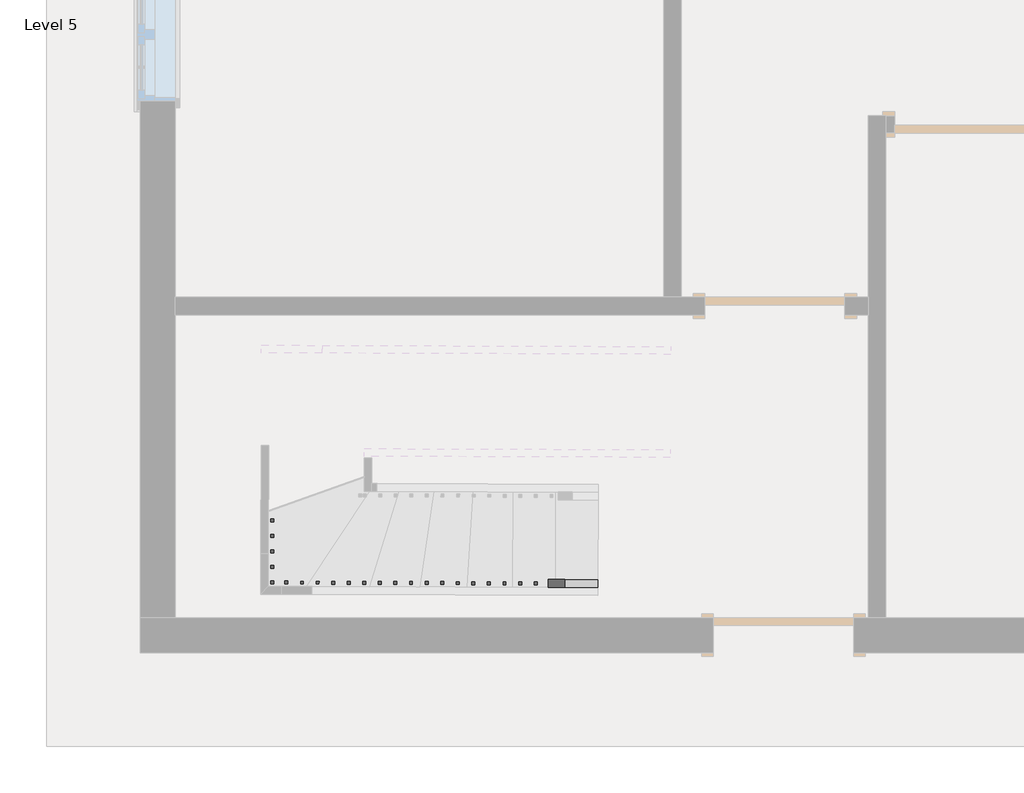
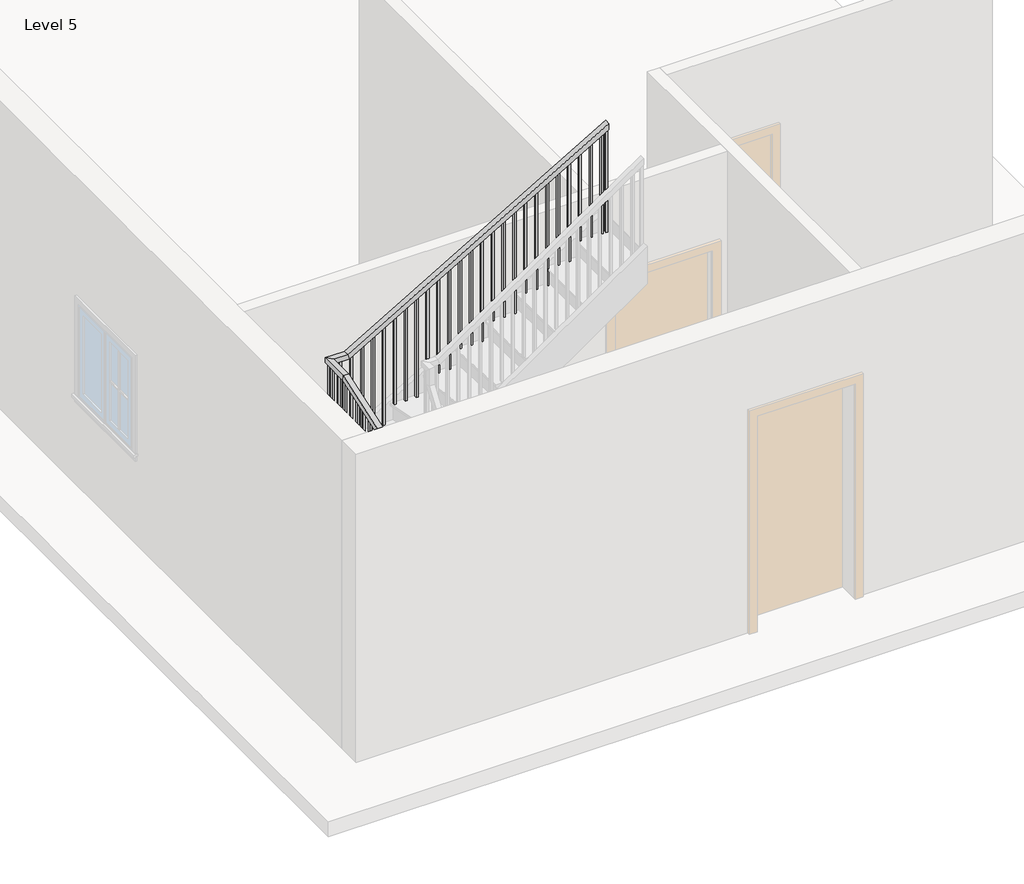
# One storey, part 2 of 3: 1 railing.
"""IFC4 building model written with IfcOpenShell, lengths in millimetres."""

from ifc_helpers import new_model, si_unit, frame, origin, place, context, project, spatial, polyline, outline, extrude, faceted_brep, element, save

model = new_model("IFC4")

# Units and contexts
model_context = context("Model", 3, world=origin())
ifc_project = project(units=[si_unit("LENGTHUNIT", "METRE", prefix="MILLI")], contexts=[model_context])

# Site, building, storey
site = spatial("IfcSite", under=ifc_project)
building = spatial("IfcBuilding", under=site)
storey = spatial("IfcBuildingStorey", under=building, Name="Level 5", Elevation=9601.2)

# Railing
placement = place(None, origin())
element("IfcRailing", 1, ObjectType="Handrail - Rectangular", at=placement, inside=storey, context=model_context, shape_type="SolidModel", body=[
    faceted_brep([(-2342.0274141, -4826.0015756, 10684.9333333), (-2342.0274141, -4826.0015756, 10627.3375993), (-2341.8555281, -4775.2018664, 10627.3375993), (-2341.8555281, -4775.2018664, 10684.9333333), (-4375.5150225, -4819.1210645, 11771.3704289), (-4388.2346185, -4819.0780265, 11720.5704289), (-4388.0627326, -4768.2783173, 11720.5704289), (-4375.3431366, -4768.3213553, 11771.3704289), (-4491.7270905, -4818.7278493, 11771.3704289), (-4491.7270905, -4818.7278493, 11720.5704289), (-4440.7554953, -4768.100026, 11720.5704289), (-4440.7554953, -4768.100026, 11771.3704289), (-4491.153576, -4649.2296115, 11771.3704289), (-4491.1254156, -4640.9069784, 11720.5704289), (-4440.3257064, -4641.0788644, 11720.5704289), (-4440.3538668, -4649.4014974, 11771.3704289), (-4487.5712496, -3590.4977417, 12127.849629), (-4487.5430892, -3582.1751086, 12077.049629), (-4436.74338, -3582.3469946, 12077.049629), (-4436.7715404, -3590.6696276, 12127.849629), (-4486.5726753, -3295.3759891, 12127.849629), (-4486.5726753, -3295.3759891, 12077.049629), (-4435.9448521, -3346.3475843, 12077.049629), (-4435.9448521, -3346.3475843, 12127.849629), (-4306.8228358, -3295.9841909, 12127.849629), (-4292.9867911, -3296.0310065, 12077.049629), (-4293.1586771, -3346.8307157, 12077.049629), (-4306.9947217, -3346.7839001, 12127.849629), (-1866.6470501, -3304.2407725, 13563.6), (-1866.8189361, -3355.0404817, 13563.6), (-1866.8189361, -3355.0404817, 13504.6591495), (-1866.6470501, -3304.2407725, 13504.6591495)], [[[0, 1, 2, 3]], [[1, 0, 4, 5]], [[2, 1, 5, 6]], [[3, 2, 6, 7]], [[0, 3, 7, 4]], [[5, 4, 8, 9]], [[6, 5, 9, 10]], [[7, 6, 10, 11]], [[4, 7, 11, 8]], [[9, 8, 12, 13]], [[10, 9, 13, 14]], [[11, 10, 14, 15]], [[8, 11, 15, 12]], [[13, 12, 16, 17]], [[14, 13, 17, 18]], [[15, 14, 18, 19]], [[12, 15, 19, 16]], [[17, 16, 20, 21]], [[18, 17, 21, 22]], [[19, 18, 22, 23]], [[16, 19, 23, 20]], [[21, 20, 24, 25]], [[22, 21, 25, 26]], [[23, 22, 26, 27]], [[20, 23, 27, 24]], [[28, 29, 30, 31]], [[25, 24, 28, 31]], [[26, 25, 31, 30]], [[27, 26, 30, 29]], [[24, 27, 29, 28]]]),
    extrude(outline(polyline([(234.2042864, 19.05), (1221.3020607, 19.05), (1221.3020607, 0.0), (222.9957135, 0.0), (234.2042864, 19.05)])), frame((-1911.7805866, -3339.0132586, 13701.1687274), z_axis=(0.0033835818014388316, 0.9999942756707125, 0.0), x_axis=(0.0, 0.0, -1.0)), (0.0, 0.0, 1.0), 19.05),
    extrude(outline(polyline([(234.2042864, 19.0499999), (1161.5230057, 19.0499999), (1161.5230057, 0.0), (222.9957136, 0.0), (234.2042864, 19.0499999)])), frame((-2013.3800051, -3338.6694867, 13641.3896724), z_axis=(0.0033835818014388316, 0.9999942756707125, 0.0), x_axis=(0.0, 0.0, -1.0)), (0.0, 0.0, 1.0), 19.05),
    extrude(outline(polyline([(234.2042864, 19.0499999), (1101.7439506, 19.0499999), (1101.7439506, 0.0), (222.9957136, 0.0), (234.2042864, 19.0499999)])), frame((-2114.9794235, -3338.3257147, 13581.6106173), z_axis=(0.0033835818014388316, 0.9999942756707125, 0.0), x_axis=(0.0, 0.0, -1.0)), (0.0, 0.0, 1.0), 19.05),
    extrude(outline(polyline([(234.2042864, 19.0499999), (1211.2982289, 19.0499999), (1211.2982289, 0.0), (222.9957135, 0.0), (234.2042864, 19.0499999)])), frame((-2216.5788419, -3337.9819428, 13521.8315622), z_axis=(0.0033835818014388316, 0.9999942756707125, 0.0), x_axis=(0.0, 0.0, -1.0)), (0.0, 0.0, 1.0), 19.05),
    extrude(outline(polyline([(234.2042864, 19.0499999), (1151.5191739, 19.0499999), (1151.5191739, 0.0), (222.9957136, 0.0), (234.2042864, 19.0499999)])), frame((-2318.1782603, -3337.6381709, 13462.0525072), z_axis=(0.0033835818014388316, 0.9999942756707125, 0.0), x_axis=(0.0, 0.0, -1.0)), (0.0, 0.0, 1.0), 19.05),
    extrude(outline(polyline([(234.2042864, 19.0499999), (1261.0734521, 19.0499999), (1261.0734521, 0.0), (222.9957136, 0.0), (234.2042864, 19.0499999)])), frame((-2419.7776787, -3337.294399, 13402.2734521), z_axis=(0.0033835818014388316, 0.9999942756707125, 0.0), x_axis=(0.0, 0.0, -1.0)), (0.0, 0.0, 1.0), 19.05),
    extrude(outline(polyline([(234.2042864, 19.0499999), (1201.294397, 19.0499999), (1201.294397, 0.0), (222.9957136, 0.0), (234.2042864, 19.0499999)])), frame((-2521.3770971, -3336.9506271, 13342.494397), z_axis=(0.0033835818014388316, 0.9999942756707125, 0.0), x_axis=(0.0, 0.0, -1.0)), (0.0, 0.0, 1.0), 19.05),
    extrude(outline(polyline([(234.2042864, 19.05), (1141.515342, 19.05), (1141.515342, 0.0), (222.9957136, 0.0), (234.2042864, 19.05)])), frame((-2622.9765155, -3336.6068552, 13282.715342), z_axis=(0.0033835818014388316, 0.9999942756707125, 0.0), x_axis=(0.0, 0.0, -1.0)), (0.0, 0.0, 1.0), 19.05),
    extrude(outline(polyline([(234.2042864, 19.05), (1251.0696202, 19.05), (1251.0696202, 0.0), (222.9957136, 0.0), (234.2042864, 19.05)])), frame((-2724.5759339, -3336.2630833, 13222.9362869), z_axis=(0.0033835818014388316, 0.9999942756707125, 0.0), x_axis=(0.0, 0.0, -1.0)), (0.0, 0.0, 1.0), 19.05),
    extrude(outline(polyline([(234.2042864, 19.05), (1191.2905651, 19.05), (1191.2905651, 0.0), (222.9957136, 0.0), (234.2042864, 19.05)])), frame((-2826.1753523, -3335.9193114, 13163.1572318), z_axis=(0.0033835818014388316, 0.9999942756707125, 0.0), x_axis=(0.0, 0.0, -1.0)), (0.0, 0.0, 1.0), 19.05),
    extrude(outline(polyline([(234.2042865, 19.05), (1131.5115101, 19.05), (1131.5115101, 0.0), (222.9957136, 0.0), (234.2042865, 19.05)])), frame((-2927.7747707, -3335.5755395, 13103.3781768), z_axis=(0.0033835818014388316, 0.9999942756707125, 0.0), x_axis=(0.0, 0.0, -1.0)), (0.0, 0.0, 1.0), 19.05),
    extrude(outline(polyline([(234.2042864, 19.05), (1241.0657884, 19.05), (1241.0657884, 0.0), (222.9957136, 0.0), (234.2042864, 19.05)])), frame((-3029.3741891, -3335.2317675, 13043.5991217), z_axis=(0.0033835818014388316, 0.9999942756707125, 0.0), x_axis=(0.0, 0.0, -1.0)), (0.0, 0.0, 1.0), 19.05),
    extrude(outline(polyline([(234.2042864, 19.05), (1181.2867333, 19.05), (1181.2867333, 0.0), (222.9957136, 0.0), (234.2042864, 19.05)])), frame((-3130.9736075, -3334.8879956, 12983.8200666), z_axis=(0.0033835818014388316, 0.9999942756707125, 0.0), x_axis=(0.0, 0.0, -1.0)), (0.0, 0.0, 1.0), 19.05),
    extrude(outline(polyline([(234.2042865, 19.0499999), (1121.5076783, 19.0499999), (1121.5076783, 0.0), (222.9957136, 0.0), (234.2042865, 19.0499999)])), frame((-3232.573026, -3334.5442237, 12924.0410116), z_axis=(0.0033835818014388316, 0.9999942756707125, 0.0), x_axis=(0.0, 0.0, -1.0)), (0.0, 0.0, 1.0), 19.05),
    extrude(outline(polyline([(234.2042864, 19.0499999), (1231.0619565, 19.0499999), (1231.0619565, 0.0), (222.9957136, 0.0), (234.2042864, 19.0499999)])), frame((-3334.1724444, -3334.2004518, 12864.2619565), z_axis=(0.0033835818014388316, 0.9999942756707125, 0.0), x_axis=(0.0, 0.0, -1.0)), (0.0, 0.0, 1.0), 19.05),
    extrude(outline(polyline([(234.2042864, 19.0499999), (1171.2829014, 19.0499999), (1171.2829014, 0.0), (222.9957136, 0.0), (234.2042864, 19.0499999)])), frame((-3435.7718628, -3333.8566799, 12804.4829014), z_axis=(0.0033835818014388316, 0.9999942756707125, 0.0), x_axis=(0.0, 0.0, -1.0)), (0.0, 0.0, 1.0), 19.05),
    extrude(outline(polyline([(234.2042864, 19.0499999), (1111.5038463, 19.0499999), (1111.5038463, 0.0), (222.9957135, 0.0), (234.2042864, 19.0499999)])), frame((-3537.3712812, -3333.512908, 12744.7038463), z_axis=(0.0033835818014388316, 0.9999942756707125, 0.0), x_axis=(0.0, 0.0, -1.0)), (0.0, 0.0, 1.0), 19.05),
    extrude(outline(polyline([(234.2042864, 19.0499999), (1221.0581246, 19.0499999), (1221.0581246, 0.0), (222.9957136, 0.0), (234.2042864, 19.0499999)])), frame((-3638.9706996, -3333.1691361, 12684.9247913), z_axis=(0.0033835818014388316, 0.9999942756707125, 0.0), x_axis=(0.0, 0.0, -1.0)), (0.0, 0.0, 1.0), 19.05),
    extrude(outline(polyline([(234.2042864, 19.0499999), (1161.2790695, 19.0499999), (1161.2790695, 0.0), (222.9957136, 0.0), (234.2042864, 19.0499999)])), frame((-3740.570118, -3332.8253642, 12625.1457362), z_axis=(0.0033835818014388316, 0.9999942756707125, 0.0), x_axis=(0.0, 0.0, -1.0)), (0.0, 0.0, 1.0), 19.05),
    extrude(outline(polyline([(234.2042864, 19.05), (1101.5000144, 19.05), (1101.5000144, 0.0), (222.9957135, 0.0), (234.2042864, 19.05)])), frame((-3842.1695364, -3332.4815923, 12565.3666811), z_axis=(0.0033835818014388316, 0.9999942756707125, 0.0), x_axis=(0.0, 0.0, -1.0)), (0.0, 0.0, 1.0), 19.05),
    extrude(outline(polyline([(234.2042864, 19.05), (1211.0542928, 19.05), (1211.0542928, 0.0), (222.9957136, 0.0), (234.2042864, 19.05)])), frame((-3943.7689548, -3332.1378203, 12505.5876261), z_axis=(0.0033835818014388316, 0.9999942756707125, 0.0), x_axis=(0.0, 0.0, -1.0)), (0.0, 0.0, 1.0), 19.05),
    extrude(outline(polyline([(234.2042864, 19.05), (1151.2752377, 19.05), (1151.2752377, 0.0), (222.9957136, 0.0), (234.2042864, 19.05)])), frame((-4045.3683732, -3331.7940484, 12445.808571), z_axis=(0.0033835818014388316, 0.9999942756707125, 0.0), x_axis=(0.0, 0.0, -1.0)), (0.0, 0.0, 1.0), 19.05),
    extrude(outline(polyline([(234.2042864, 19.05), (1091.4961826, 19.05), (1091.4961826, 0.0), (222.9957136, 0.0), (234.2042864, 19.05)])), frame((-4146.9677916, -3331.4502765, 12386.0295159), z_axis=(0.0033835818014388316, 0.9999942756707125, 0.0), x_axis=(0.0, 0.0, -1.0)), (0.0, 0.0, 1.0), 19.05),
    extrude(outline(polyline([(234.2042865, 19.05), (1031.7171276, 19.05), (1031.7171276, 0.0), (222.9957136, 0.0), (234.2042865, 19.05)])), frame((-4248.56721, -3331.1065046, 12326.2504609), z_axis=(0.0033835818014388316, 0.9999942756707125, 0.0), x_axis=(0.0, 0.0, -1.0)), (0.0, 0.0, 1.0), 19.05),
    extrude(outline(polyline([(-4369.1520622, -3311.6483845), (-4350.1021712, -3311.7128418), (-4350.1666284, -3330.7627327), (-4369.2165194, -3330.6982755), (-4369.1520622, -3311.6483845)])), frame((0.0, 0.0, 11294.5333333), z_axis=(0.0, 0.0, 1.0), x_axis=(1.0, 0.0, 0.0)), (0.0, 0.0, 1.0), 782.5162957),
    extrude(outline(polyline([(-4470.9856602, -3380.5147968), (-4470.921203, -3361.4649058), (-4451.871312, -3361.5293631), (-4451.9357693, -3380.579254), (-4470.9856602, -3380.5147968)])), frame((0.0, 0.0, 11294.5333333), z_axis=(0.0, 0.0, 1.0), x_axis=(1.0, 0.0, 0.0)), (0.0, 0.0, 1.0), 782.5162957),
    extrude(outline(polyline([(-4471.3294321, -3482.1142152), (-4471.2649749, -3463.0643242), (-4452.215084, -3463.1287815), (-4452.2795412, -3482.1786724), (-4471.3294321, -3482.1142152)])), frame((0.0, 0.0, 11125.2), z_axis=(0.0, 0.0, 1.0), x_axis=(1.0, 0.0, 0.0)), (0.0, 0.0, 1.0), 951.849629),
    extrude(outline(polyline([(-4471.6732041, -3583.7136336), (-4471.6087468, -3564.6637426), (-4452.5588559, -3564.7281999), (-4452.6233131, -3583.7780908), (-4471.6732041, -3583.7136336)])), frame((0.0, 0.0, 11125.2), z_axis=(0.0, 0.0, 1.0), x_axis=(1.0, 0.0, 0.0)), (0.0, 0.0, 1.0), 951.849629),
    extrude(outline(polyline([(231.8070867, 19.0499999), (1148.9478489, 19.0499999), (1148.9478489, 0.0), (225.3929132, 0.0), (231.8070867, 19.0499999)])), frame((-4452.9026278, -3666.3276183, 12274.1478489), z_axis=(-0.9999942756707125, 0.003383581801438912, 0.0), x_axis=(0.0, 0.0, -1.0)), (0.0, 0.0, 1.0), 19.05),
    extrude(outline(polyline([(231.8070868, 19.0499999), (1114.7389237, 19.0499999), (1114.7389237, 0.0), (225.3929133, 0.0), (231.8070868, 19.0499999)])), frame((-4453.2463997, -3767.9270367, 12239.9389237), z_axis=(-0.9999942756707125, 0.003383581801438912, 0.0), x_axis=(0.0, 0.0, -1.0)), (0.0, 0.0, 1.0), 19.05),
    extrude(outline(polyline([(231.8070867, 19.0499999), (1080.5299984, 19.0499999), (1080.5299984, 0.0), (225.3929132, 0.0), (231.8070867, 19.0499999)])), frame((-4453.5901716, -3869.5264551, 12205.7299984), z_axis=(-0.9999942756707125, 0.003383581801438912, 0.0), x_axis=(0.0, 0.0, -1.0)), (0.0, 0.0, 1.0), 19.05),
    extrude(outline(polyline([(231.8070867, 19.05), (1215.6544064, 19.05), (1215.6544064, 0.0), (225.3929132, 0.0), (231.8070867, 19.05)])), frame((-4453.9339435, -3971.1258735, 12171.5210731), z_axis=(-0.9999942756707125, 0.003383581801438912, 0.0), x_axis=(0.0, 0.0, -1.0)), (0.0, 0.0, 1.0), 19.05),
    extrude(outline(polyline([(231.8070868, 19.05), (1181.4454812, 19.05), (1181.4454812, 0.0), (225.3929133, 0.0), (231.8070868, 19.05)])), frame((-4454.2777154, -4072.7252919, 12137.3121479), z_axis=(-0.9999942756707125, 0.003383581801438912, 0.0), x_axis=(0.0, 0.0, -1.0)), (0.0, 0.0, 1.0), 19.05),
    extrude(outline(polyline([(231.8070867, 19.05), (1147.2365559, 19.05), (1147.2365559, 0.0), (225.3929132, 0.0), (231.8070867, 19.05)])), frame((-4454.6214873, -4174.3247103, 12103.1032226), z_axis=(-0.9999942756707125, 0.003383581801438912, 0.0), x_axis=(0.0, 0.0, -1.0)), (0.0, 0.0, 1.0), 19.05),
    extrude(outline(polyline([(231.8070868, 19.05), (1113.0276307, 19.05), (1113.0276307, 0.0), (225.3929133, 0.0), (231.8070868, 19.05)])), frame((-4454.9652592, -4275.9241287, 12068.8942974), z_axis=(-0.9999942756707125, 0.003383581801438912, 0.0), x_axis=(0.0, 0.0, -1.0)), (0.0, 0.0, 1.0), 19.05),
    extrude(outline(polyline([(231.8070868, 19.05), (1248.1520388, 19.05), (1248.1520388, 0.0), (225.3929133, 0.0), (231.8070868, 19.05)])), frame((-4455.3090312, -4377.5235471, 12034.6853721), z_axis=(-0.9999942756707125, 0.003383581801438912, 0.0), x_axis=(0.0, 0.0, -1.0)), (0.0, 0.0, 1.0), 19.05),
    extrude(outline(polyline([(231.8070867, 19.05), (1213.9431135, 19.05), (1213.9431135, 0.0), (225.3929132, 0.0), (231.8070867, 19.05)])), frame((-4455.6528031, -4479.1229655, 12000.4764468), z_axis=(-0.9999942756707125, 0.003383581801438912, 0.0), x_axis=(0.0, 0.0, -1.0)), (0.0, 0.0, 1.0), 19.05),
    extrude(outline(polyline([(231.8070868, 19.0499999), (1179.7341883, 19.0499999), (1179.7341883, 0.0), (225.3929133, 0.0), (231.8070868, 19.0499999)])), frame((-4455.996575, -4580.722384, 11966.2675216), z_axis=(-0.9999942756707125, 0.003383581801438912, 0.0), x_axis=(0.0, 0.0, -1.0)), (0.0, 0.0, 1.0), 19.05),
    extrude(outline(polyline([(-4475.4546951, -4701.3072361), (-4475.3902378, -4682.2573451), (-4456.3403469, -4682.3218024), (-4456.4048041, -4701.3716933), (-4475.4546951, -4701.3072361)])), frame((0.0, 0.0, 10786.5333333), z_axis=(0.0, 0.0, 1.0), x_axis=(1.0, 0.0, 0.0)), (0.0, 0.0, 1.0), 934.0370956),
    extrude(outline(polyline([(223.5110808, 19.05), (1155.0403583, 19.05), (1155.0403583, 0.0), (233.6889192, 0.0), (223.5110808, 19.05)])), frame((-4364.4371224, -4803.2834569, 11941.5736916), z_axis=(0.0033835818014387046, 0.9999942756707125, 0.0), x_axis=(0.0, 0.0, -1.0)), (0.0, 0.0, 1.0), 19.05),
    extrude(outline(polyline([(223.5110808, 19.05), (1100.7585537, 19.05), (1100.7585537, 0.0), (233.6889192, 0.0), (223.5110808, 19.05)])), frame((-4262.837704, -4803.6272288, 11887.291887), z_axis=(0.0033835818014387046, 0.9999942756707125, 0.0), x_axis=(0.0, 0.0, -1.0)), (0.0, 0.0, 1.0), 19.05),
    extrude(outline(polyline([(223.5110808, 19.05), (1215.8100824, 19.05), (1215.8100824, 0.0), (233.6889192, 0.0), (223.5110808, 19.05)])), frame((-4161.2382856, -4803.9710007, 11833.0100824), z_axis=(0.0033835818014387046, 0.9999942756707125, 0.0), x_axis=(0.0, 0.0, -1.0)), (0.0, 0.0, 1.0), 19.05),
    extrude(outline(polyline([(223.5110809, 19.0499999), (1161.5282778, 19.0499999), (1161.5282778, 0.0), (233.6889192, 0.0), (223.5110809, 19.0499999)])), frame((-4059.6388672, -4804.3147726, 11778.7282778), z_axis=(0.0033835818014387046, 0.9999942756707125, 0.0), x_axis=(0.0, 0.0, -1.0)), (0.0, 0.0, 1.0), 19.05),
    extrude(outline(polyline([(223.5110808, 19.0499999), (1107.2464731, 19.0499999), (1107.2464731, 0.0), (233.6889191, 0.0), (223.5110808, 19.0499999)])), frame((-3958.0394488, -4804.6585445, 11724.4464731), z_axis=(0.0033835818014387046, 0.9999942756707125, 0.0), x_axis=(0.0, 0.0, -1.0)), (0.0, 0.0, 1.0), 19.05),
    extrude(outline(polyline([(223.5110808, 19.0499999), (1052.9646685, 19.0499999), (1052.9646685, 0.0), (233.6889192, 0.0), (223.5110808, 19.0499999)])), frame((-3856.4400304, -4805.0023164, 11670.1646685), z_axis=(0.0033835818014387046, 0.9999942756707125, 0.0), x_axis=(0.0, 0.0, -1.0)), (0.0, 0.0, 1.0), 19.05),
    extrude(outline(polyline([(223.5110808, 19.0499999), (1168.0161972, 19.0499999), (1168.0161972, 0.0), (233.6889192, 0.0), (223.5110808, 19.0499999)])), frame((-3754.840612, -4805.3460883, 11615.8828639), z_axis=(0.0033835818014387046, 0.9999942756707125, 0.0), x_axis=(0.0, 0.0, -1.0)), (0.0, 0.0, 1.0), 19.05),
    extrude(outline(polyline([(223.5110808, 19.0499999), (1113.7343926, 19.0499999), (1113.7343926, 0.0), (233.6889192, 0.0), (223.5110808, 19.0499999)])), frame((-3653.2411936, -4805.6898602, 11561.6010593), z_axis=(0.0033835818014387046, 0.9999942756707125, 0.0), x_axis=(0.0, 0.0, -1.0)), (0.0, 0.0, 1.0), 19.05),
    extrude(outline(polyline([(223.5110808, 19.0499999), (1059.452588, 19.0499999), (1059.452588, 0.0), (233.6889192, 0.0), (223.5110808, 19.0499999)])), frame((-3551.6417752, -4806.0336322, 11507.3192547), z_axis=(0.0033835818014387046, 0.9999942756707125, 0.0), x_axis=(0.0, 0.0, -1.0)), (0.0, 0.0, 1.0), 19.05),
    extrude(outline(polyline([(223.5110808, 19.05), (1174.5041168, 19.05), (1174.5041168, 0.0), (233.6889192, 0.0), (223.5110808, 19.05)])), frame((-3450.0423567, -4806.3774041, 11453.0374501), z_axis=(0.0033835818014387046, 0.9999942756707125, 0.0), x_axis=(0.0, 0.0, -1.0)), (0.0, 0.0, 1.0), 19.05),
    extrude(outline(polyline([(223.5110809, 19.05), (1120.2223122, 19.05), (1120.2223122, 0.0), (233.6889192, 0.0), (223.5110809, 19.05)])), frame((-3348.4429383, -4806.721176, 11398.7556455), z_axis=(0.0033835818014387046, 0.9999942756707125, 0.0), x_axis=(0.0, 0.0, -1.0)), (0.0, 0.0, 1.0), 19.05),
    extrude(outline(polyline([(223.5110808, 19.05), (1065.9405075, 19.05), (1065.9405075, 0.0), (233.6889191, 0.0), (223.5110808, 19.05)])), frame((-3246.8435199, -4807.0649479, 11344.4738408), z_axis=(0.0033835818014387046, 0.9999942756707125, 0.0), x_axis=(0.0, 0.0, -1.0)), (0.0, 0.0, 1.0), 19.05),
    extrude(outline(polyline([(223.5110808, 19.05), (1180.9920362, 19.05), (1180.9920362, 0.0), (233.6889192, 0.0), (223.5110808, 19.05)])), frame((-3145.2441015, -4807.4087198, 11290.1920362), z_axis=(0.0033835818014387046, 0.9999942756707125, 0.0), x_axis=(0.0, 0.0, -1.0)), (0.0, 0.0, 1.0), 19.05),
    extrude(outline(polyline([(223.5110808, 19.05), (1126.7102316, 19.05), (1126.7102316, 0.0), (233.6889192, 0.0), (223.5110808, 19.05)])), frame((-3043.6446831, -4807.7524917, 11235.9102316), z_axis=(0.0033835818014387046, 0.9999942756707125, 0.0), x_axis=(0.0, 0.0, -1.0)), (0.0, 0.0, 1.0), 19.05),
    extrude(outline(polyline([(223.5110808, 19.05), (1072.428427, 19.05), (1072.428427, 0.0), (233.6889192, 0.0), (223.5110808, 19.05)])), frame((-2942.0452647, -4808.0962636, 11181.628427), z_axis=(0.0033835818014387046, 0.9999942756707125, 0.0), x_axis=(0.0, 0.0, -1.0)), (0.0, 0.0, 1.0), 19.05),
    extrude(outline(polyline([(223.5110808, 19.05), (1187.4799557, 19.05), (1187.4799557, 0.0), (233.6889192, 0.0), (223.5110808, 19.05)])), frame((-2840.4458463, -4808.4400355, 11127.3466224), z_axis=(0.0033835818014387046, 0.9999942756707125, 0.0), x_axis=(0.0, 0.0, -1.0)), (0.0, 0.0, 1.0), 19.05),
    extrude(outline(polyline([(223.5110809, 19.0499999), (1133.1981511, 19.0499999), (1133.1981511, 0.0), (233.6889192, 0.0), (223.5110809, 19.0499999)])), frame((-2738.8464279, -4808.7838074, 11073.0648178), z_axis=(0.0033835818014387046, 0.9999942756707125, 0.0), x_axis=(0.0, 0.0, -1.0)), (0.0, 0.0, 1.0), 19.05),
    extrude(outline(polyline([(223.5110809, 19.0499999), (1078.9163465, 19.0499999), (1078.9163465, 0.0), (233.6889192, 0.0), (223.5110809, 19.0499999)])), frame((-2637.2470095, -4809.1275794, 11018.7830132), z_axis=(0.0033835818014387046, 0.9999942756707125, 0.0), x_axis=(0.0, 0.0, -1.0)), (0.0, 0.0, 1.0), 19.05),
    extrude(outline(polyline([(223.5110808, 19.0499999), (1193.9678752, 19.0499999), (1193.9678752, 0.0), (233.6889191, 0.0), (223.5110808, 19.0499999)])), frame((-2535.6475911, -4809.4713513, 10964.5012085), z_axis=(0.0033835818014387046, 0.9999942756707125, 0.0), x_axis=(0.0, 0.0, -1.0)), (0.0, 0.0, 1.0), 19.05),
    extrude(outline(polyline([(223.5110808, 19.0499999), (1139.6860706, 19.0499999), (1139.6860706, 0.0), (233.6889192, 0.0), (223.5110808, 19.0499999)])), frame((-2434.0481727, -4809.8151232, 10910.2194039), z_axis=(0.0033835818014387046, 0.9999942756707125, 0.0), x_axis=(0.0, 0.0, -1.0)), (0.0, 0.0, 1.0), 19.05),
    extrude(outline(polyline([(-4470.8159378, -3330.3545036), (-4470.7514806, -3311.3046126), (-4451.7015896, -3311.3690698), (-4451.7660469, -3330.4189608), (-4470.8159378, -3330.3545036)])), frame((0.0, 0.0, 11294.5333333), z_axis=(0.0, 0.0, 1.0), x_axis=(1.0, 0.0, 0.0)), (0.0, 0.0, 1.0), 782.5162957),
    extrude(outline(polyline([(-4456.748576, -4802.9711117), (-4475.798467, -4802.9066545), (-4475.7340098, -4783.8567635), (-4456.6841188, -4783.9212208), (-4456.748576, -4802.9711117)])), frame((0.0, 0.0, 10786.5333333), z_axis=(0.0, 0.0, 1.0), x_axis=(1.0, 0.0, 0.0)), (0.0, 0.0, 1.0), 934.0370956),
    extrude(outline(polyline([(234.2042864, 19.05), (1247.7881964, 19.05), (1247.7881964, 0.0), (222.9957136, 0.0), (234.2042864, 19.05)])), frame((-1866.7652217, -3339.1655726, 13727.6548631), z_axis=(0.0033835818014388316, 0.9999942756707125, 0.0), x_axis=(0.0, 0.0, -1.0)), (0.0, 0.0, 1.0), 19.05),
    extrude(outline(polyline([(223.5110808, 19.05), (1090.4931852, 19.05), (1090.4931852, 0.0), (233.6889192, 0.0), (223.5110808, 19.05)])), frame((-2341.9736997, -4810.1266665, 10861.0265185), z_axis=(0.0033835818014387046, 0.9999942756707125, 0.0), x_axis=(0.0, 0.0, -1.0)), (0.0, 0.0, 1.0), 19.05),
])

save(model, "model.ifc")

# Revit data of these elements
# Type "Handrail - Rectangular"
#   Assembly Code = "C2010400"
#   built-in parameter 1008612 = 0.0416667 (stored number, unit not read)
#   built-in parameter 1008611 = 0.0416667 (stored number, unit not read)
#   built-in parameter 1008609 = 0.333333 (stored number, unit not read)
#   built-in parameter 1008604 = 0.166667 (stored number, unit not read)
#   built-in parameter 1008603 = 0.166667 (stored number, unit not read)
#   Railing Height = 3' - 0"
#   built-in parameter 1008630 = 2
#   built-in parameter 1008610 = 2
#   built-in parameter 1008618 = Baluster - Square : 3/4"
# Element 1 (IfcRailing, "Handrail - Rectangular")
#   Phase Created = New Construction
